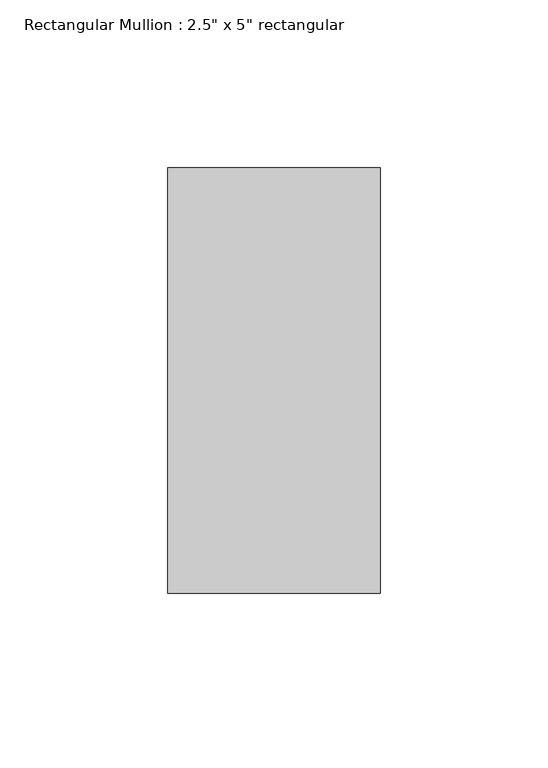
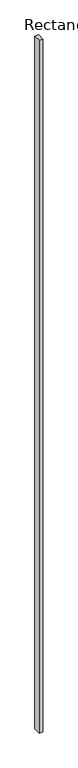
"""IFC4 building model written with IfcOpenShell, lengths in millimetres: member geometry."""

from ifc_helpers import new_model, si_unit, frame, origin, place, context, project, spatial, polyline, outline, extrude, source, transform, mapped, element, save


def member_943fafd7(model_context):
    return source(origin(), model_context, "Body", "SweptSolid", [
        extrude(outline(polyline([(0.0, 63.5), (0.0, -63.5), (-63.5, -63.5), (-63.5, 63.5), (0.0, 63.5)])), frame((0.0, 0.0, -12619.0552746), z_axis=(0.0, 0.0, 1.0), x_axis=(1.0, 0.0, 0.0)), (0.0, 0.0, 1.0), 12619.0552746),
    ])


if __name__ == "__main__":
    model = new_model("IFC4")
    model_context = context("Model", 3, world=origin())
    ifc_project = project(units=[si_unit("LENGTHUNIT", "METRE", prefix="MILLI")], contexts=[model_context])
    site = spatial("IfcSite", under=ifc_project)
    building = spatial("IfcBuilding", under=site)
    placement = place(None, origin())
    member_shape = member_943fafd7(model_context)
    element("IfcMember", 1, ObjectType="Rectangular Mullion : 2.5\" x 5\" rectangular", at=placement, inside=building, context=model_context, shape_type="MappedRepresentation", body=[
        mapped(member_shape, transform((0.0, 0.0, 0.0), x_axis=(1.0, 0.0, 0.0), y_axis=(0.0, 1.0, 0.0), z_axis=(0.0, 0.0, 1.0))),
    ])
    save(model, "model.ifc")

# Revit data of these elements
# Type "Rectangular Mullion : 2.5\" x 5\" rectangular"
#   built-in parameter 1007304 = 0.416667 (stored number, unit not read)
#   built-in parameter 1007301 = 0.104167 (stored number, unit not read)
#   built-in parameter 1007300 = 0.104167 (stored number, unit not read)
# Element 1 (IfcMember, "Rectangular Mullion : 2.5\" x 5\" rectangular")
#   Materials on its faces: "Aluminum"
# Materials
#   "Aluminum": class "Metal", colour RGB 247 247 247, transparency 0, Description = "Aluminum 6061", Cost = 0
